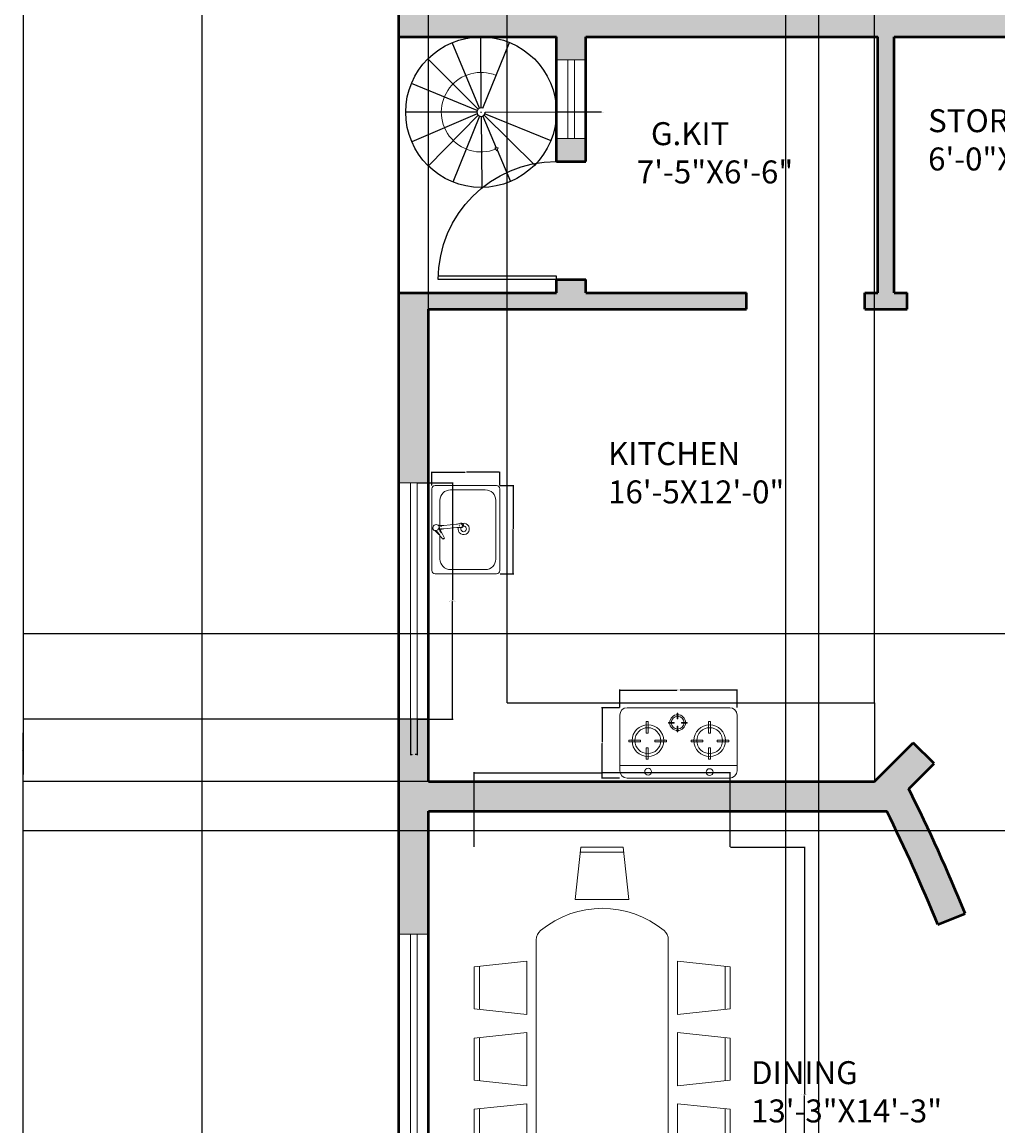
# Model space of a CAD drawing. Units: inches. Extents: x 134045 to 134755, y 144691 to 145880.
# Tile 3 of 6: x 134045 to 134343, y 145178 to 145515. Entities that reach past the tile are written whole.
import ezdxf

# ---------------------------------------------------------------- set-up
doc = ezdxf.new("R2010")
doc.units = ezdxf.units.IN
for name, color, linetype, lineweight in [('A-ANNO-DIMS', 2, 'Continuous', 18), ('A-ANNO-SYMB', 7, 'Continuous', 18), ('A-AREA-IDEN', 7, 'Continuous', 18), ('A-DOOR', 4, 'Continuous', 25), ('A-EQPM', 9, 'Continuous', 18), ('A-FLOR-CASE', 8, 'Continuous', 25), ('A-FLOR-FIXT', 9, 'Continuous', 18), ('A-FLOR-STRS', 7, 'Continuous', 25), ('A-FLOR-STRS-PATT', 252, 'Continuous', 13), ('A-FURN', 8, 'Continuous', 18), ('A-GLAZ', 4, 'Continuous', 18), ('A-WALL', 7, 'Continuous', 50), ('A-WALL-PATT', 252, 'Continuous', 13), ('C-PROP', 7, 'Continuous', 25)]:
    doc.layers.add(name, color=color, linetype=linetype, lineweight=lineweight)
doc.styles.get("Standard").update_dxf_attribs({"font": 'arial.ttf'})
doc.dimstyles.get("Standard").update_dxf_attribs({"dimtxt": 0.18, "dimasz": 0.18, "dimexe": 0.18, "dimexo": 0.0625, "dimgap": 0.09, "dimtad": 0, "dimtih": 1, "dimtoh": 1, "dimdec": 4, "dimzin": 0, "dimdsep": 46, "dimtxsty": 'Standard', "dimcen": 0.09, "dimadec": 0, "dimazin": 0, "dimtfac": 1, "dimtdec": 4, "dimtofl": 0, "dimtmove": 0, "dimatfit": 3, "dimfxl": 1, "dimtolj": 1, "dimtzin": 0, "dimarcsym": 0})

# ---------------------------------------------------------------- blocks, each defined once
blk = doc.blocks.new('A$C113D154D')
for p, q in [((0.96, 1.7118), (1.0076, 2.1547)), ((1.0076, 2.1547), (1.3624, 2.1547)), ((1.3624, 2.1547), (1.41, 1.7118)), ((1.56, 1.7118), (1.6076, 2.1547)), ((1.6076, 2.1547), (1.9624, 2.1547)), ((1.9624, 2.1547), (2.01, 1.7118)), ((2.16, 1.7118), (2.2076, 2.1547)), ((2.2076, 2.1547), (2.5624, 2.1547)), ((2.5624, 2.1547), (2.61, 1.7118)), ((2.76, 1.7118), (2.8076, 2.1547)), ((2.8076, 2.1547), (3.1624, 2.1547)), ((3.1624, 2.1547), (3.21, 1.7118)), ((1.003, 2.1119), (1.367, 2.1119)), ((1.603, 2.1119), (1.967, 2.1119)), ((2.203, 2.1119), (2.567, 2.1119)), ((2.803, 2.1119), (3.167, 2.1119)), ((1.41, 1.7118), (0.96, 1.7118)), ((2.01, 1.7118), (1.56, 1.7118)), ((2.61, 1.7118), (2.16, 1.7118)), ((3.21, 1.7118), (2.76, 1.7118)), ((0.7802, 1.6333), (3.3898, 1.6333)), ((0, 1.2523), (0.4429, 1.2999)), ((0, 0.8975), (0, 1.2523)), ((0.0429, 0.8929), (0.0429, 1.2569)), ((0.4429, 1.2999), (0.4429, 0.8499)), ((3.7271, 1.2999), (3.7271, 0.8499)), ((4.17, 1.2523), (3.7271, 1.2999)), ((4.1272, 0.8929), (4.1272, 1.2569)), ((4.17, 0.8975), (4.17, 1.2523)), ((0.4429, 0.8499), (0, 0.8975)), ((3.7271, 0.8499), (4.17, 0.8975)), ((3.3898, 0.5214), (0.7802, 0.5214)), ((1.41, 0.4429), (0.96, 0.4429)), ((0.96, 0.4429), (1.0076, 0)), ((1.3624, 0), (1.41, 0.4429)), ((2.01, 0.4429), (1.56, 0.4429)), ((1.56, 0.4429), (1.6076, 0)), ((1.9624, 0), (2.01, 0.4429)), ((2.61, 0.4429), (2.16, 0.4429)), ((2.16, 0.4429), (2.2076, 0)), ((2.5624, 0), (2.61, 0.4429)), ((3.21, 0.4429), (2.76, 0.4429)), ((2.76, 0.4429), (2.8076, 0)), ((3.1624, 0), (3.21, 0.4429)), ((1.003, 0.0429), (1.367, 0.0429)), ((1.0076, 0), (1.3624, 0)), ((1.603, 0.0429), (1.967, 0.0429)), ((1.6076, 0), (1.9624, 0)), ((2.203, 0.0429), (2.567, 0.0429)), ((2.2076, 0), (2.5624, 0)), ((2.803, 0.0429), (3.167, 0.0429)), ((2.8076, 0), (3.1624, 0))]:
    blk.add_line(p, q)
for centre, radius, start, end in [((1.3313, 1.0774), 0.8152, 140.39755, 219.60245), ((0.7802, 1.5333), 0.1, 90, 140.39755), ((3.3898, 1.5333), 0.1, 39.60245, 90), ((2.8387, 1.0774), 0.8152, 320.39755, 39.60245), ((0.7802, 0.6214), 0.1, 219.60245, 270), ((3.3898, 0.6214), 0.1, 270, 320.39755)]:
    blk.add_arc(centre, radius, start, end)
blk = doc.blocks.new('A$C1B254B08')
for p, q in [((20, 414.5), (278.5, 414.5)), ((278.5, 414.5), (518, 414.5)), ((0, 20), (0, 394.5)), ((90.2, 364.5), (232.9, 364.5)), ((275, 340.3), (282.6, 261.9)), ((303, 263.9), (295.5, 341.4)), ((296.4, 364.5), (447.8, 364.5)), ((538, 394.5), (538, 20)), ((26.2, 88.5), (26.2, 300.5)), ((511.8, 300.5), (511.8, 88.5)), ((447.8, 24.5), (90.2, 24.5)), ((518, 0), (20, 0))]:
    blk.add_line(p, q)
for centre, radius, start, end in [((20, 394.5), 20, 90, 180), ((280.7, 388), 20, 287.37848, 143.44123), ((518, 394.5), 20, 0, 90), ((90.2, 300.5), 64, 90, 180), ((218.4, 343.7), 6.64, 127.29995, 303.51976), ((59.9, 551.8), 255, 307.29995, 323.44123), ((220.3, 343.9), 4.91, 158.92924, 241.9125), ((362.9, 125.6), 255, 107.37848, 123.51976), ((189.9, 438.1), 86.6, 305.66886, 327.17012), ((298.2, 285.8), 86.6, 103.6496, 125.15085), ((280, 388.4), 16.2, 164.00843, 277.23501), ((175.5, 330.4), 100, 5.6774, 19.04527), ((246.9, 349.5), 29.3, 4.17107, 27.91331), ((320.7, 356.3), 29.3, 157.81042, 186.31744), ((395, 351.3), 100, 162.19035, 185.67746), ((447.8, 300.5), 64, 0, 90), ((273.7, 220.2), 34.6, 74.3543, 12.13808), ((273.7, 220.2), 16.8, 61.4601, 4.85789), ((295.6, 234.6), 13.9, 171.17496, 20.1799), ((183.1, 252), 100, 351.17496, 5.6774), ((295.7, 235), 8.12, 213.71984, 15.80061), ((295.2, 239.5), 7.59, 64.48838, 123.74119), ((402.5, 273.8), 100, 185.67746, 200.1799), ((90.2, 88.5), 64, 180, 270), ((447.8, 88.5), 64, 270, 0), ((20, 20), 20, 180, 270), ((518, 20), 20, 270, 0)]:
    blk.add_arc(centre, radius, start, end)
blk = doc.blocks.new('A$C2A3C6842')
for p, q in [((45, 432), (675, 432)), ((0, 45), (0, 387)), ((161.8, 346.9), (173.2, 346.9)), ((161.8, 275.6), (161.8, 346.9)), ((173.2, 346.9), (173.2, 275.6)), ((298.4, 341.9), (298.4, 336.2)), ((334, 341.9), (298.4, 341.9)), ((334, 336.2), (334, 341.9)), ((351.6, 363.3), (351.6, 398.9)), ((351.6, 398.9), (357.3, 398.9)), ((357.3, 363.3), (351.6, 363.3)), ((357.3, 398.9), (357.3, 363.3)), ((378.5, 336.2), (378.5, 341.9)), ((378.5, 341.9), (414.2, 341.9)), ((414.2, 341.9), (414.2, 336.2)), ((544.7, 346.9), (556.1, 346.9)), ((544.7, 275.6), (544.7, 346.9)), ((556.1, 346.9), (556.1, 275.6)), ((720, 387), (720, 45)), ((173.2, 275.6), (161.8, 275.6)), ((298.4, 336.2), (334, 336.2)), ((357.3, 318.8), (351.6, 318.8)), ((351.6, 318.8), (351.6, 283.1)), ((351.6, 283.1), (357.3, 283.1)), ((357.3, 283.1), (357.3, 318.8)), ((414.2, 336.2), (378.5, 336.2)), ((556.1, 275.6), (544.7, 275.6)), ((55.3, 232.9), (55.3, 221.5)), ((126.6, 232.9), (55.3, 232.9)), ((55.3, 221.5), (126.6, 221.5)), ((126.6, 221.5), (126.6, 232.9)), ((215.6, 221.5), (215.6, 232.9)), ((215.6, 232.9), (286.9, 232.9)), ((286.9, 221.5), (215.6, 221.5)), ((286.9, 232.9), (286.9, 221.5)), ((438.2, 232.9), (438.2, 221.5)), ((509.5, 232.9), (438.2, 232.9)), ((438.2, 221.5), (509.5, 221.5)), ((509.5, 221.5), (509.5, 232.9)), ((598.5, 232.9), (669.8, 232.9)), ((598.5, 221.5), (598.5, 232.9)), ((669.8, 221.5), (598.5, 221.5)), ((669.8, 232.9), (669.8, 221.5)), ((173.2, 186.6), (161.8, 186.6)), ((161.8, 186.6), (161.8, 115.3)), ((173.2, 115.3), (173.2, 186.6)), ((556.1, 186.6), (544.7, 186.6)), ((544.7, 186.6), (544.7, 115.3)), ((556.1, 115.3), (556.1, 186.6)), ((1.2, 76.7), (719.9, 76.7)), ((161.8, 115.3), (173.2, 115.3)), ((544.7, 115.3), (556.1, 115.3)), ((675, 0), (45, 0))]:
    blk.add_line(p, q)
at = {"extrusion": (0, -1e-16, -1)}
for centre, major_axis, start_param, end_param in [((45, 387), (31.8, 31.8), 3.926991, 5.497787), ((172.2, 229.8), (-97.3, 0.1), -0.001099, 6.282086), ((551.8, 229.8), (-97.3, 0.1), -0.001099, 6.282086), ((173.7, 39), (-14.8, 14.8), 5.497787, 11.780972)]:
    blk.add_ellipse(centre, major_axis=major_axis, ratio=1, start_param=start_param, end_param=end_param, dxfattribs=at)
at = {"extrusion": (0, 1e-16, -1)}
blk.add_ellipse((675, 387), major_axis=(-31.8, 31.8), ratio=1, start_param=0.785398, end_param=2.356194, dxfattribs=at)
at = {"extrusion": (-1e-16, -1e-16, -1)}
blk.add_ellipse((355.1, 340.4), major_axis=(48.7, 0.1), ratio=1, start_param=3.144125, end_param=9.42731, dxfattribs=at)
at = {"extrusion": (-1e-16, 0, -1)}
for centre, major_axis, start_param, end_param in [((355.1, 340.4), (-39.7, 0), -0.000334, 6.282851), ((45, 45), (-31.8, 31.8), 3.926991, 5.497787)]:
    blk.add_ellipse(centre, major_axis=major_axis, ratio=1, start_param=start_param, end_param=end_param, dxfattribs=at)
at = {"extrusion": (-1e-16, -4e-16, -1)}
for centre in [(172.2, 229.8), (551.8, 229.8)]:
    blk.add_ellipse(centre, major_axis=(-79.3, 0), ratio=1, start_param=-0.0002116186602152, end_param=6.282973688519371, dxfattribs=at)
at = {"extrusion": (2e-16, -2e-16, -1)}
blk.add_ellipse((551.4, 36.4), major_axis=(14.8, 14.8), ratio=1, start_param=3.926991, end_param=10.210176, dxfattribs=at)
at = {"extrusion": (-2e-16, 1e-16, -1)}
blk.add_ellipse((675, 45), major_axis=(31.8, 31.8), ratio=1, start_param=0.785398, end_param=2.356194, dxfattribs=at)
at = {"text_generation_flag": 4, "flags": 9}
for tag in ['XSIZE', 'YSIZE']:
    blk.add_attdef(tag, (361.3, 264.9), '', height=0.45, rotation=180, dxfattribs=at)
blk = doc.blocks.new('DOOR-SWING-36IN')
for p, q in [((0, 1), (35.99, 1)), ((0, 0), (0, 1)), ((0, 0), (36, 0))]:
    blk.add_line(p, q)
blk.add_arc((0, 0), 36, 0, 90)
blk = doc.blocks.new('WIN-GLAZ-24IN')
for p, q in [((0, 0), (0, 24)), ((2, 0), (2, 24))]:
    blk.add_line(p, q)
blk = doc.blocks.new('WIN-GLAZ-72IN')
for p, q in [((0, 72), (0, 0)), ((2, 72), (2, 0))]:
    blk.add_line(p, q)
blk = doc.blocks.new('WIN-GLAZ-96IN')
for p, q in [((0, 0), (0, 96)), ((2, 0), (2, 96))]:
    blk.add_line(p, q)
blk = doc.blocks.new('*D30')
at = {"layer": 'A-ANNO-DIMS', "color": 0, "lineweight": -2, "transparency": 16777216}
for p, q in [((134165.67, 145374.42), (134176.58, 145374.42)), ((134176.4, 145374.24), (134176.4, 145338.61)), ((134176.4, 145302.6), (134176.4, 145338.24)), ((134165.67, 145302.42), (134176.58, 145302.42))]:
    blk.add_line(p, q, dxfattribs=at)
at = {"layer": 'A-ANNO-DIMS', "color": 0, "transparency": 16777216}
for points in [[(134176.37, 145374.24), (134176.43, 145374.24), (134176.4, 145374.42)], [(134176.37, 145302.6), (134176.43, 145302.6), (134176.4, 145302.42)]]:
    blk.add_solid(points, dxfattribs=at)
at = {"layer": 'Defpoints', "color": 0, "transparency": 16777216}
for p in [(134165.6, 145374.42), (134176.4, 145374.42), (134165.6, 145302.42)]:
    blk.add_point(p, dxfattribs=at)
at = {"layer": 'A-ANNO-DIMS', "color": 0, "transparency": 16777216, "insert": (134176.4, 145338.42), "char_height": 0.18, "attachment_point": 5}
blk.add_mtext('\\A1;WINDOW 72 TYP.', dxfattribs=at)
blk = doc.blocks.new('*D31')
at = {"layer": 'A-ANNO-DIMS', "color": 0, "lineweight": -2, "transparency": 16777216}
for p, q in [((134163.6, 145302.36), (134163.6, 145291.44)), ((134165.6, 145302.36), (134165.6, 145291.44)), ((134163.78, 145291.62), (134164.14, 145291.62)), ((134165.42, 145291.62), (134165.06, 145291.62))]:
    blk.add_line(p, q, dxfattribs=at)
at = {"layer": 'A-ANNO-DIMS', "color": 0, "transparency": 16777216}
for points in [[(134163.78, 145291.65), (134163.78, 145291.59), (134163.6, 145291.62)], [(134165.42, 145291.65), (134165.42, 145291.59), (134165.6, 145291.62)]]:
    blk.add_solid(points, dxfattribs=at)
at = {"layer": 'Defpoints', "color": 0, "transparency": 16777216}
for p in [(134163.6, 145302.42), (134165.6, 145302.42), (134165.6, 145291.62)]:
    blk.add_point(p, dxfattribs=at)
at = {"layer": 'A-ANNO-DIMS', "color": 0, "transparency": 16777216, "insert": (134164.6, 145291.62), "char_height": 0.18, "attachment_point": 5}
blk.add_mtext('\\A1;2 TYP.', dxfattribs=at)
blk = doc.blocks.new('*D40')
at = {"layer": 'A-ANNO-DIMS', "color": 0, "lineweight": -2, "transparency": 16777216}
for p, q in [((134261.18, 145263.4), (134283.96, 145263.4)), ((134283.78, 145263.22), (134283.78, 145188.06)), ((134283.78, 145112.53), (134283.78, 145187.69)), ((134261.18, 145112.35), (134283.96, 145112.35))]:
    blk.add_line(p, q, dxfattribs=at)
at = {"layer": 'A-ANNO-DIMS', "color": 0, "transparency": 16777216}
for points in [[(134283.75, 145263.22), (134283.81, 145263.22), (134283.78, 145263.4)], [(134283.75, 145112.53), (134283.81, 145112.53), (134283.78, 145112.35)]]:
    blk.add_solid(points, dxfattribs=at)
at = {"layer": 'Defpoints', "color": 0, "transparency": 16777216}
for p in [(134261.12, 145263.4), (134261.12, 145112.35), (134283.78, 145112.35)]:
    blk.add_point(p, dxfattribs=at)
at = {"layer": 'A-ANNO-DIMS', "color": 0, "transparency": 16777216, "insert": (134283.78, 145187.88), "char_height": 0.18, "attachment_point": 5}
blk.add_mtext('\\A1;DINING SET 151', dxfattribs=at)
blk = doc.blocks.new('*D41')
at = {"layer": 'A-ANNO-DIMS', "color": 0, "lineweight": -2, "transparency": 16777216}
for p, q in [((134183.07, 145263.47), (134183.07, 145286.24)), ((134183.25, 145286.06), (134221.88, 145286.06)), ((134260.94, 145286.06), (134222.31, 145286.06)), ((134261.12, 145263.47), (134261.12, 145286.24))]:
    blk.add_line(p, q, dxfattribs=at)
at = {"layer": 'A-ANNO-DIMS', "color": 0, "transparency": 16777216}
for points in [[(134183.25, 145286.09), (134183.25, 145286.03), (134183.07, 145286.06)], [(134260.94, 145286.09), (134260.94, 145286.03), (134261.12, 145286.06)]]:
    blk.add_solid(points, dxfattribs=at)
at = {"layer": 'Defpoints', "color": 0, "transparency": 16777216}
for p in [(134261.12, 145286.06), (134183.07, 145263.4), (134261.12, 145263.4)]:
    blk.add_point(p, dxfattribs=at)
at = {"layer": 'A-ANNO-DIMS', "color": 0, "transparency": 16777216, "insert": (134222.09, 145286.06), "char_height": 0.18, "attachment_point": 5}
blk.add_mtext('\\A1;78', dxfattribs=at)
blk = doc.blocks.new('*D42')
at = {"layer": 'A-ANNO-DIMS', "color": 0, "lineweight": -2, "transparency": 16777216}
for p, q in [((134190.92, 145373.59), (134195.08, 145373.59)), ((134194.9, 145373.41), (134194.9, 145360.31)), ((134194.9, 145346.83), (134194.9, 145359.94)), ((134190.92, 145346.65), (134195.08, 145346.65))]:
    blk.add_line(p, q, dxfattribs=at)
at = {"layer": 'A-ANNO-DIMS', "color": 0, "transparency": 16777216}
for points in [[(134194.87, 145373.41), (134194.93, 145373.41), (134194.9, 145373.59)], [(134194.87, 145346.83), (134194.93, 145346.83), (134194.9, 145346.65)]]:
    blk.add_solid(points, dxfattribs=at)
at = {"layer": 'Defpoints', "color": 0, "transparency": 16777216}
for p in [(134190.86, 145373.59), (134194.9, 145373.59), (134190.86, 145346.65)]:
    blk.add_point(p, dxfattribs=at)
at = {"layer": 'A-ANNO-DIMS', "color": 0, "transparency": 16777216, "insert": (134194.9, 145360.12), "char_height": 0.18, "attachment_point": 5}
blk.add_mtext('\\A1;SINK 27', dxfattribs=at)
blk = doc.blocks.new('*D43')
at = {"layer": 'A-ANNO-DIMS', "color": 0, "lineweight": -2, "transparency": 16777216}
for p, q in [((134170.1, 145373.65), (134170.1, 145377.81)), ((134170.28, 145377.63), (134180.28, 145377.63)), ((134190.68, 145377.63), (134180.68, 145377.63)), ((134190.86, 145373.65), (134190.86, 145377.81))]:
    blk.add_line(p, q, dxfattribs=at)
at = {"layer": 'A-ANNO-DIMS', "color": 0, "transparency": 16777216}
for points in [[(134170.28, 145377.66), (134170.28, 145377.6), (134170.1, 145377.63)], [(134190.68, 145377.66), (134190.68, 145377.6), (134190.86, 145377.63)]]:
    blk.add_solid(points, dxfattribs=at)
at = {"layer": 'Defpoints', "color": 0, "transparency": 16777216}
for p in [(134170.1, 145377.63), (134170.1, 145373.59), (134190.86, 145373.59)]:
    blk.add_point(p, dxfattribs=at)
at = {"layer": 'A-ANNO-DIMS', "color": 0, "transparency": 16777216, "insert": (134180.48, 145377.63), "char_height": 0.18, "attachment_point": 5}
blk.add_mtext('\\A1;21', dxfattribs=at)
blk = doc.blocks.new('*D44')
at = {"layer": 'A-ANNO-DIMS', "color": 0, "lineweight": -2, "transparency": 16777216}
for p, q in [((134227.44, 145305.93), (134227.44, 145311.41)), ((134227.62, 145311.23), (134244.79, 145311.23)), ((134263.01, 145311.23), (134245.84, 145311.23)), ((134263.19, 145305.93), (134263.19, 145311.41))]:
    blk.add_line(p, q, dxfattribs=at)
at = {"layer": 'A-ANNO-DIMS', "color": 0, "transparency": 16777216}
for points in [[(134227.62, 145311.26), (134227.62, 145311.2), (134227.44, 145311.23)], [(134263.01, 145311.26), (134263.01, 145311.2), (134263.19, 145311.23)]]:
    blk.add_solid(points, dxfattribs=at)
at = {"layer": 'Defpoints', "color": 0, "transparency": 16777216}
for p in [(134263.19, 145311.23), (134227.44, 145305.86), (134263.19, 145305.86)]:
    blk.add_point(p, dxfattribs=at)
at = {"layer": 'A-ANNO-DIMS', "color": 0, "transparency": 16777216, "insert": (134245.32, 145311.23), "char_height": 0.18, "attachment_point": 5}
blk.add_mtext('\\A1;HOB 36', dxfattribs=at)
blk = doc.blocks.new('*D45')
at = {"layer": 'A-ANNO-DIMS', "color": 0, "lineweight": -2, "transparency": 16777216}
for p, q in [((134227.38, 145305.86), (134221.9, 145305.86)), ((134222.08, 145305.68), (134222.08, 145295.32)), ((134222.08, 145284.6), (134222.08, 145294.96)), ((134227.38, 145284.42), (134221.9, 145284.42))]:
    blk.add_line(p, q, dxfattribs=at)
at = {"layer": 'A-ANNO-DIMS', "color": 0, "transparency": 16777216}
for points in [[(134222.05, 145305.68), (134222.11, 145305.68), (134222.08, 145305.86)], [(134222.05, 145284.6), (134222.11, 145284.6), (134222.08, 145284.42)]]:
    blk.add_solid(points, dxfattribs=at)
at = {"layer": 'Defpoints', "color": 0, "transparency": 16777216}
for p in [(134222.08, 145305.86), (134227.44, 145305.86), (134227.44, 145284.42)]:
    blk.add_point(p, dxfattribs=at)
at = {"layer": 'A-ANNO-DIMS', "color": 0, "transparency": 16777216, "insert": (134222.08, 145295.14), "char_height": 0.18, "attachment_point": 5}
blk.add_mtext('\\A1;21', dxfattribs=at)
blk = doc.blocks.new('*D47')
at = {"layer": 'A-ANNO-DIMS', "color": 0, "lineweight": -2, "transparency": 16777216}
for p, q in [((134100.04, 145825.38), (134045.37, 145825.38)), ((134045.55, 145825.2), (134045.55, 145285.56)), ((134045.55, 144745.56), (134045.55, 145285.19)), ((134100.04, 144745.38), (134045.37, 144745.38))]:
    blk.add_line(p, q, dxfattribs=at)
at = {"layer": 'A-ANNO-DIMS', "color": 0, "transparency": 16777216}
for points in [[(134045.52, 145825.2), (134045.58, 145825.2), (134045.55, 145825.38)], [(134045.52, 144745.56), (134045.58, 144745.56), (134045.55, 144745.38)]]:
    blk.add_solid(points, dxfattribs=at)
at = {"layer": 'Defpoints', "color": 0, "transparency": 16777216}
for p in [(134045.55, 145825.38), (134100.1, 145825.38), (134100.1, 144745.38)]:
    blk.add_point(p, dxfattribs=at)
at = {"layer": 'A-ANNO-DIMS', "color": 0, "transparency": 16777216, "insert": (134045.55, 145285.38), "char_height": 0.18, "attachment_point": 5}
blk.add_mtext('\\A1;1080', dxfattribs=at)
blk = doc.blocks.new('*D55')
at = {"layer": 'A-ANNO-DIMS', "color": 0, "lineweight": -2, "transparency": 16777216}
for p, q in [((134278.1, 145094.44), (134278.1, 145880.11)), ((134278.28, 145879.93), (134282.89, 145879.93)), ((134287.92, 145879.93), (134283.31, 145879.93)), ((134288.1, 145094.44), (134288.1, 145880.11))]:
    blk.add_line(p, q, dxfattribs=at)
at = {"layer": 'A-ANNO-DIMS', "color": 0, "transparency": 16777216}
for points in [[(134278.28, 145879.96), (134278.28, 145879.9), (134278.1, 145879.93)], [(134287.92, 145879.96), (134287.92, 145879.9), (134288.1, 145879.93)]]:
    blk.add_solid(points, dxfattribs=at)
at = {"layer": 'Defpoints', "color": 0, "transparency": 16777216}
for p in [(134288.1, 145879.93), (134278.1, 145094.38), (134288.1, 145094.38)]:
    blk.add_point(p, dxfattribs=at)
at = {"layer": 'A-ANNO-DIMS', "color": 0, "transparency": 16777216, "insert": (134283.1, 145879.93), "char_height": 0.18, "attachment_point": 5}
blk.add_mtext('\\A1;10', dxfattribs=at)
blk = doc.blocks.new('*D61')
at = {"layer": 'A-ANNO-DIMS', "color": 0, "lineweight": -2, "transparency": 16777216}
for p, q in [((134499.04, 145328.38), (134045.37, 145328.38)), ((134045.55, 145328.2), (134045.55, 145298.56)), ((134045.55, 145268.56), (134045.55, 145298.19)), ((134439.04, 145268.38), (134045.37, 145268.38))]:
    blk.add_line(p, q, dxfattribs=at)
at = {"layer": 'A-ANNO-DIMS', "color": 0, "transparency": 16777216}
for points in [[(134045.52, 145328.2), (134045.58, 145328.2), (134045.55, 145328.38)], [(134045.52, 145268.56), (134045.58, 145268.56), (134045.55, 145268.38)]]:
    blk.add_solid(points, dxfattribs=at)
at = {"layer": 'Defpoints', "color": 0, "transparency": 16777216}
for p in [(134045.55, 145328.38), (134499.1, 145328.38), (134439.1, 145268.38)]:
    blk.add_point(p, dxfattribs=at)
at = {"layer": 'A-ANNO-DIMS', "color": 0, "transparency": 16777216, "insert": (134045.55, 145298.38), "char_height": 0.18, "attachment_point": 5}
blk.add_mtext('\\A1;60', dxfattribs=at)
blk = doc.blocks.new('*D71')
at = {"layer": 'A-ANNO-DIMS', "color": 0, "lineweight": -2, "transparency": 16777216}
for p, q in [((134169.1, 145283.44), (134169.1, 145880.11)), ((134169.28, 145879.93), (134180.88, 145879.93)), ((134192.92, 145879.93), (134181.32, 145879.93)), ((134193.1, 145307.44), (134193.1, 145880.11))]:
    blk.add_line(p, q, dxfattribs=at)
at = {"layer": 'A-ANNO-DIMS', "color": 0, "transparency": 16777216}
for points in [[(134169.28, 145879.96), (134169.28, 145879.9), (134169.1, 145879.93)], [(134192.92, 145879.96), (134192.92, 145879.9), (134193.1, 145879.93)]]:
    blk.add_solid(points, dxfattribs=at)
at = {"layer": 'Defpoints', "color": 0, "transparency": 16777216}
for p in [(134193.1, 145879.93), (134193.1, 145307.38), (134169.1, 145283.38)]:
    blk.add_point(p, dxfattribs=at)
at = {"layer": 'A-ANNO-DIMS', "color": 0, "transparency": 16777216, "insert": (134181.1, 145879.93), "char_height": 0.18, "attachment_point": 5}
blk.add_mtext('\\A1;24', dxfattribs=at)
blk = doc.blocks.new('*D72')
at = {"layer": 'A-ANNO-DIMS', "color": 0, "lineweight": -2, "transparency": 16777216}
for p, q in [((134193.1, 145307.44), (134193.1, 145880.11)), ((134193.28, 145879.93), (134248.82, 145879.93)), ((134304.92, 145879.93), (134249.38, 145879.93)), ((134305.1, 145307.44), (134305.1, 145880.11))]:
    blk.add_line(p, q, dxfattribs=at)
at = {"layer": 'A-ANNO-DIMS', "color": 0, "transparency": 16777216}
for points in [[(134193.28, 145879.96), (134193.28, 145879.9), (134193.1, 145879.93)], [(134304.92, 145879.96), (134304.92, 145879.9), (134305.1, 145879.93)]]:
    blk.add_solid(points, dxfattribs=at)
at = {"layer": 'Defpoints', "color": 0, "transparency": 16777216}
for p in [(134305.1, 145879.93), (134193.1, 145307.38), (134305.1, 145307.38)]:
    blk.add_point(p, dxfattribs=at)
at = {"layer": 'A-ANNO-DIMS', "color": 0, "transparency": 16777216, "insert": (134249.1, 145879.93), "char_height": 0.18, "attachment_point": 5}
blk.add_mtext('\\A1;112', dxfattribs=at)
blk = doc.blocks.new('*D75')
at = {"layer": 'A-ANNO-DIMS', "color": 0, "lineweight": -2, "transparency": 16777216}
for p, q in [((134169.04, 145302.42), (134045.37, 145302.42)), ((134045.55, 145302.24), (134045.55, 145293.08)), ((134045.55, 145283.56), (134045.55, 145292.72)), ((134169.04, 145283.38), (134045.37, 145283.38))]:
    blk.add_line(p, q, dxfattribs=at)
at = {"layer": 'A-ANNO-DIMS', "color": 0, "transparency": 16777216}
for points in [[(134045.52, 145302.24), (134045.58, 145302.24), (134045.55, 145302.42)], [(134045.52, 145283.56), (134045.58, 145283.56), (134045.55, 145283.38)]]:
    blk.add_solid(points, dxfattribs=at)
at = {"layer": 'Defpoints', "color": 0, "transparency": 16777216}
for p in [(134045.55, 145302.42), (134169.1, 145302.42), (134169.1, 145283.38)]:
    blk.add_point(p, dxfattribs=at)
at = {"layer": 'A-ANNO-DIMS', "color": 0, "transparency": 16777216, "insert": (134045.55, 145292.9), "char_height": 0.18, "attachment_point": 5}
blk.add_mtext('\\A1;19.047', dxfattribs=at)
blk = doc.blocks.new('*D83')
at = {"layer": 'A-ANNO-DIMS', "color": 0, "lineweight": -2, "transparency": 16777216}
for p, q in [((134185.05, 145487.41), (134185.23, 145487.41)), ((134185.14, 145487.32), (134185.14, 145487.5)), ((134221.88, 145487.41), (134208.28, 145487.41))]:
    blk.add_line(p, q, dxfattribs=at)
at = {"layer": 'A-ANNO-DIMS', "color": 0, "transparency": 16777216}
blk.add_solid([(134208.28, 145487.44), (134208.28, 145487.38), (134208.1, 145487.41)], dxfattribs=at)
at = {"layer": 'Defpoints', "color": 0, "transparency": 16777216}
for p in [(134162.18, 145487.41), (134208.1, 145487.41)]:
    blk.add_point(p, dxfattribs=at)
at = {"layer": 'A-ANNO-DIMS', "color": 0, "transparency": 16777216, "insert": (134222.37, 145487.41), "char_height": 0.18, "attachment_point": 5}
blk.add_mtext('\\A1;∅45.93', dxfattribs=at)

msp = doc.modelspace()

# ---------------------------------------------------------------- hatches: boundary and pattern name
at = {"layer": 'A-FLOR-STRS-PATT'}
h = msp.add_hatch(dxfattribs=at)
h.set_pattern_fill('ANGLE', color=256)
h.set_pattern_definition([(0, (0, 0), (0, 6.985), [5.08, -1.905]), (90, (0, 0), (-6.985, 4e-16), [5.08, -1.905])])
h.paths.add_polyline_path([(134190.3591, 145476.5617), (134189.3624, 145476.5112), (134189.9045, 145475.6732)])
at = {"layer": 'A-WALL-PATT'}
h = msp.add_hatch(color=256, dxfattribs=at)
h.dxf.hatch_style = 1
h.paths.add_polyline_path([(134169.1037, 145427.3753), (134266.1037, 145427.3753), (134266.1037, 145432.3753), (134217.1037, 145432.3753), (134217.1037, 145436.3753), (134208.1037, 145436.3753), (134208.1037, 145432.3753), (134160.1037, 145432.3753), (134160.1037, 145374.4227), (134169.1037, 145374.4227)], flags=17)
h.paths.add_polyline_path([(134217.1037, 145479.3753), (134208.1037, 145479.3753), (134208.1037, 145472.3753), (134217.1037, 145472.3753)], flags=17)
h.paths.add_polyline_path([(134217.1037, 145510.3753), (134306.1037, 145510.3753), (134306.1037, 145432.3753), (134302.1037, 145432.3753), (134302.1037, 145427.3753), (134315.1037, 145427.3753), (134315.1037, 145432.3753), (134311.1037, 145432.3753), (134311.1037, 145510.3753), (134383.1037, 145510.3753), (134383.1037, 145432.3753), (134351.1037, 145432.3753), (134351.1037, 145427.3753), (134365.1037, 145427.3753), (134365.1037, 145343.3753), (134350.8634, 145329.135), (134357.2273, 145322.771), (134364.9677, 145330.5114), (134378.8831, 145316.5959), (134385.2471, 145322.9598), (134371.3316, 145336.8753), (134374.1037, 145339.6474), (134374.1037, 145427.3753), (134392.1037, 145427.3753), (134392.1037, 145519.3753), (134358.1037, 145519.3753), (134358.1037, 145523.3753), (134349.1037, 145523.3753), (134349.1037, 145519.3753), (134169.1037, 145519.3753), (134169.1037, 145549.3753), (134160.1037, 145549.3753), (134160.1037, 145510.3753), (134208.1037, 145510.3753), (134208.1037, 145503.3753), (134217.1037, 145503.3753)])
h = msp.add_hatch(color=256, dxfattribs=at)
h.dxf.hatch_style = 1
h.paths.add_polyline_path([(134315.5458, 145281.0895), (134323.2862, 145288.8299), (134316.9222, 145295.1938), (134305.1037, 145283.3753), (134169.1037, 145283.3753), (134169.1037, 145302.4227), (134160.1037, 145302.4227), (134160.1037, 145236.8753), (134169.1037, 145236.8753), (134169.1037, 145274.3753), (134308.8316, 145274.3753, -0.01816061), (134324.3593, 145239.7695), (134332.6989, 145243.1534, 0.01959752)])

# ---------------------------------------------------------------- linework, layer by layer
at = {"layer": 'A-ANNO-SYMB'}
msp.add_lwpolyline([(134190.3591, 145476.5617), (134189.3624, 145476.5112), (134189.9045, 145475.6732)], close=True, dxfattribs=at)
msp.add_arc((134185.1406, 145487.4122), 12.1261, 67.719607, 291.598106, dxfattribs=at)
at = {"layer": 'A-FLOR-CASE'}
for p, q in [((134193.1037, 145307.3753), (134193.1037, 145427.3753)), ((134193.1037, 145307.3753), (134305.1037, 145307.3753)), ((134305.1037, 145307.3753), (134305.1037, 145283.3753))]:
    msp.add_line(p, q, dxfattribs=at)
at = {"layer": 'A-FLOR-STRS'}
for p, q in [((134185.1366, 145488.7012), (134185.0702, 145510.3752)), ((134184.6446, 145488.6019), (134176.3042, 145508.6071)), ((134185.6293, 145488.605), (134193.8468, 145508.6609)), ((134184.2277, 145488.3223), (134168.8783, 145503.6247)), ((134183.9493, 145487.9046), (134163.9187, 145496.1835)), ((134183.8516, 145487.4122), (134162.1774, 145487.4122)), ((134183.9554, 145486.9052), (134164.0278, 145478.3812)), ((134184.2389, 145486.491), (134169.0784, 145471.0015)), ((134184.6592, 145486.2164), (134176.5648, 145466.1105)), ((134185.1524, 145486.1232), (134185.3518, 145464.45)), ((134185.6439, 145486.2255), (134189.7555, 145476.5311)), ((134186.059, 145486.5077), (134201.502, 145471.2997)), ((134186.3348, 145486.9271), (134206.4159, 145478.7712)), ((134186.4296, 145487.4201), (134208.1033, 145487.553)), ((134190.022, 145475.9029), (134194.1068, 145466.2719))]:
    msp.add_line(p, q, dxfattribs=at)
msp.add_circle((134185.1406, 145487.4122), 22.9631, dxfattribs=at)
msp.add_arc((134185.1406, 145487.4122), 1.289, 67.719607, 0.351372, dxfattribs=at)
at = {"layer": 'A-GLAZ'}
for p, q in [((134217.1037, 145503.3753), (134208.1037, 145503.3753)), ((134217.1037, 145479.3753), (134208.1037, 145479.3753)), ((134169.1037, 145374.4227), (134160.1037, 145374.4227)), ((134169.1037, 145302.4227), (134160.1037, 145302.4227)), ((134169.1037, 145236.8753), (134160.1037, 145236.8753))]:
    msp.add_line(p, q, dxfattribs=at)
at = {"layer": 'A-WALL'}
for p, q in [((134160.1037, 145094.3753), (134160.1037, 145765.3753)), ((134160.1037, 145510.3753), (134208.1037, 145510.3753)), ((134208.1037, 145472.3753), (134208.1037, 145510.3753)), ((134217.1037, 145510.3753), (134306.1037, 145510.3753)), ((134217.1037, 145472.3753), (134217.1037, 145510.3753)), ((134306.1037, 145432.3753), (134306.1037, 145510.3753)), ((134311.1037, 145432.3753), (134311.1037, 145510.3753)), ((134311.1037, 145510.3753), (134383.1037, 145510.3753)), ((134208.1037, 145472.3753), (134217.1037, 145472.3753)), ((134208.1037, 145432.3753), (134208.1037, 145436.3753)), ((134208.1037, 145436.3753), (134217.1037, 145436.3753)), ((134217.1037, 145432.3753), (134217.1037, 145436.3753)), ((134160.1037, 145432.3753), (134208.1037, 145432.3753)), ((134217.1037, 145432.3753), (134266.1037, 145432.3753)), ((134266.1037, 145427.3753), (134266.1037, 145432.3753)), ((134302.1037, 145427.3753), (134302.1037, 145432.3753)), ((134302.1037, 145432.3753), (134306.1037, 145432.3753)), ((134311.1037, 145432.3753), (134315.1037, 145432.3753)), ((134315.1037, 145427.3753), (134315.1037, 145432.3753)), ((134169.1037, 145427.3753), (134266.1037, 145427.3753)), ((134169.1037, 145283.3753), (134169.1037, 145427.3753)), ((134302.1037, 145427.3753), (134315.1037, 145427.3753)), ((134305.1037, 145283.3753), (134316.9222, 145295.1938)), ((134323.2862, 145288.8299), (134316.9222, 145295.1938)), ((134315.5458, 145281.0895), (134323.2862, 145288.8299)), ((134169.1037, 145283.3753), (134305.1037, 145283.3753)), ((134169.1037, 145274.3753), (134308.8316, 145274.3753)), ((134169.1037, 145103.3753), (134169.1037, 145274.3753)), ((134324.3593, 145239.7695), (134332.6989, 145243.1534))]:
    msp.add_line(p, q, dxfattribs=at)
for radius, end in [(531.3157, 26.575845), (522.3157, 26.246647)]:
    msp.add_arc((133840.3674, 145043.3884), radius, 22.084999, end, dxfattribs=at)
at = {"layer": 'C-PROP'}
msp.add_line((134100.1037, 144745.3753), (134100.1037, 145825.3753), dxfattribs=at)

# ---------------------------------------------------------------- block references
at = {"layer": 'A-DOOR', "extrusion": (0, 0, -1), "zscale": -1}
msp.add_blockref('DOOR-SWING-36IN', (-134208.1034, 145436.375), dxfattribs=at)
at = {"layer": 'A-EQPM', "xscale": 0.0496421835922516, "yscale": 0.0496421835922516, "zscale": 0.0496421835922516}
msp.add_blockref('A$C2A3C6842', (134227.4444, 145284.4183), dxfattribs=at)
at = {"layer": 'A-FLOR-FIXT', "xscale": 0.0500722032276694, "yscale": 0.0500722032276694, "zscale": 0.0500722032276694, "rotation": 90}
msp.add_blockref('A$C1B254B08', (134190.8579, 145346.6522), dxfattribs=at)
at = {"layer": 'A-FURN', "xscale": 36.22436829030262, "yscale": 36.22436829030262, "zscale": 36.22436829030262, "rotation": 270}
msp.add_blockref('A$C113D154D', (134183.0679, 145263.4031), dxfattribs=at)
at = {"layer": 'A-GLAZ'}
for name, p in [('WIN-GLAZ-24IN', (134211.604, 145479.375)), ('WIN-GLAZ-72IN', (134163.604, 145302.423)), ('WIN-GLAZ-96IN', (134163.604, 145140.875))]:
    msp.add_blockref(name, p, dxfattribs=at)

# ---------------------------------------------------------------- texts
at = {"layer": 'A-AREA-IDEN', "char_height": 7, "attachment_point": 1}
for s, width, insert in [('STORE\\P6\'-0"X6\'-6"', 40.020524, (134321.4449, 145488.3122)), ('  G.KIT\\P7\'-5"X6\'-6"', 63.365833, (134232.6494, 145484.3547)), ('KITCHEN\\P16\'-5X12\'-0"', 62.240081, (134223.8628, 145386.817)), ('DINING\\P13\'-3"X14\'-3"', 46.210983, (134267.4431, 145198.1133))]:
    msp.add_mtext_dynamic_manual_height_columns(s, width=width, gutter_width=12.5, heights=[0], dxfattribs=dict(at, insert=insert))

# ---------------------------------------------------------------- dimensions: what is measured, and where the dimension line sits
at = {"layer": 'A-ANNO-DIMS'}
for base, p1, p2, picture, middle in [((134193.1037, 145879.9253), (134169.1037, 145283.3753), (134193.1037, 145307.3753), '*D71', (134181.1037, 145879.9253)), ((134305.1037, 145879.9253), (134193.1037, 145307.3753), (134305.1037, 145307.3753), '*D72', (134249.1037, 145879.9253)), ((134288.1037, 145879.9253), (134278.1037, 145094.3753), (134288.1037, 145094.3753), '*D55', (134283.1037, 145879.9253)), ((134261.121, 145286.0615), (134183.0679, 145263.4031), (134261.121, 145263.4031), '*D41', (134222.0944, 145286.0615))]:
    dim = msp.add_linear_dim(base=base, p1=p1, p2=p2, dimstyle='Standard', override={"dimdec": 0, "dimlfac": 1, "dimrnd": 0, "dimzin": 0, "dimdsep": 46, "dimlunit": 2}, dxfattribs=at)
    dim.commit()
    dim.dimension.update_dxf_attribs({"geometry": picture, "text_midpoint": middle})
for base, p1, p2, angle, override, picture, middle in [((134045.5537, 145825.3753), (134100.1037, 144745.3753), (134100.1037, 145825.3753), 90, {"dimdec": 0, "dimlfac": 1, "dimrnd": 0, "dimzin": 0, "dimdsep": 46, "dimlunit": 2}, '*D47', (134045.5537, 145285.3753)), ((134170.1047, 145377.6331), (134190.8579, 145373.5921), (134170.1047, 145373.5921), 180, {"dimdec": 0, "dimlfac": 1, "dimrnd": 0, "dimzin": 0, "dimdsep": 46, "dimlunit": 2}, '*D43', (134180.4813, 145377.6331)), ((134045.5537, 145328.3753), (134439.1037, 145268.3753), (134499.1037, 145328.3753), 90, {"dimdec": 0, "dimlfac": 1, "dimrnd": 0, "dimzin": 0, "dimdsep": 46, "dimlunit": 2}, '*D61', (134045.5537, 145298.3753)), ((134222.0831, 145305.8637), (134227.4444, 145284.4183), (134227.4444, 145305.8637), 90, {"dimdec": 0, "dimlfac": 1, "dimrnd": 0, "dimzin": 0, "dimdsep": 46, "dimlunit": 2}, '*D45', (134222.0831, 145295.141)), ((134045.5537, 145302.4227), (134169.1037, 145283.3753), (134169.1037, 145302.4227), 90, {"dimdec": 3, "dimlfac": 1, "dimrnd": 0, "dimzin": 0, "dimdsep": 46, "dimlunit": 2}, '*D75', (134045.5537, 145292.899))]:
    dim = msp.add_linear_dim(base=base, p1=p1, p2=p2, angle=angle, dimstyle='Standard', override=override, dxfattribs=at)
    dim.commit()
    dim.dimension.update_dxf_attribs({"geometry": picture, "text_midpoint": middle})
dim = msp.add_diameter_dim_2p(p1=(134162.1774, 145487.4124), p2=(134208.1037, 145487.412), dimstyle='Standard', override={"dimdec": 2, "dimlfac": 1, "dimrnd": 0, "dimzin": 0, "dimdsep": 46, "dimlunit": 2}, dxfattribs=at)
dim.commit()
dim.dimension.update_dxf_attribs({"geometry": '*D83', "text_midpoint": (134221.8816, 145487.4119), "dimtype": 163})
for base, p1, p2, angle, text, picture, middle in [((134176.4037, 145374.4227), (134165.6037, 145302.4227), (134165.6037, 145374.4227), 90, 'WINDOW <> TYP.', '*D30', (134176.4037, 145338.4227)), ((134194.8989, 145373.5921), (134190.8579, 145346.6522), (134190.8579, 145373.5921), 90, 'SINK <>', '*D42', (134194.8989, 145360.1221)), ((134283.7794, 145112.3471), (134261.121, 145263.4031), (134261.121, 145112.3471), 270, 'DINING SET <>', '*D40', (134283.7794, 145187.8751))]:
    dim = msp.add_linear_dim(base=base, p1=p1, p2=p2, angle=angle, text=text, dimstyle='Standard', override={"dimdec": 0, "dimlfac": 1, "dimrnd": 0, "dimzin": 0, "dimdsep": 46, "dimlunit": 2}, dxfattribs=at)
    dim.commit()
    dim.dimension.update_dxf_attribs({"geometry": picture, "text_midpoint": middle})
for base, p1, p2, text, picture, middle in [((134263.1868, 145311.2251), (134227.4444, 145305.8637), (134263.1868, 145305.8637), 'HOB <>', '*D44', (134245.3156, 145311.2251)), ((134165.6037, 145291.6227), (134163.6037, 145302.4227), (134165.6037, 145302.4227), '<> TYP.', '*D31', (134164.6037, 145291.6227))]:
    dim = msp.add_linear_dim(base=base, p1=p1, p2=p2, text=text, dimstyle='Standard', override={"dimdec": 0, "dimlfac": 1, "dimrnd": 0, "dimzin": 0, "dimdsep": 46, "dimlunit": 2}, dxfattribs=at)
    dim.commit()
    dim.dimension.update_dxf_attribs({"geometry": picture, "text_midpoint": middle})

doc.saveas('drawing.dxf')
